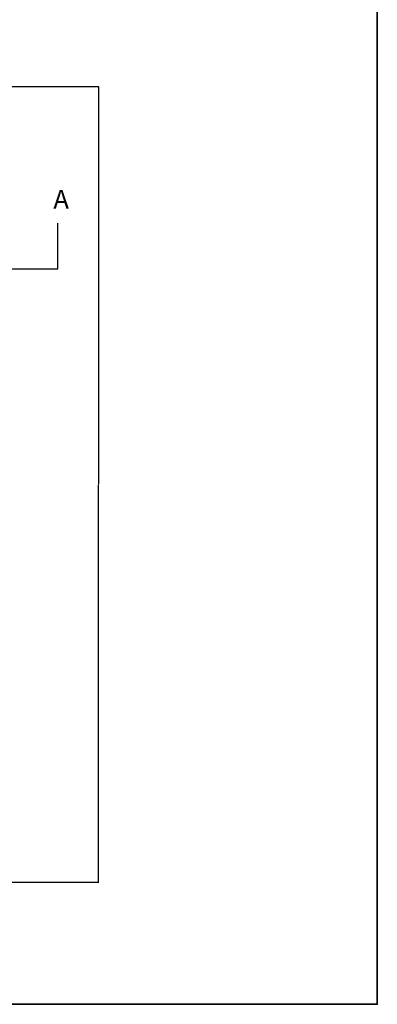
# Model space of a CAD drawing. Units: inches. Extents: x 1832 to 2989, y 1644 to 2902.
# Tile 6 of 8: x 2760 to 2989, y 1644 to 2272. Entities that reach past the tile are written whole.
import ezdxf

# ---------------------------------------------------------------- set-up
doc = ezdxf.new("R2010")
doc.units = ezdxf.units.IN
for name, color, linetype, lineweight in [('A-ANNO-DIMS', 2, 'Continuous', 18), ('A-ANNO-SYMB', 3, 'Continuous', 25), ('A-ANNO-TTLB', 7, 'Continuous', 35)]:
    doc.layers.add(name, color=color, linetype=linetype, lineweight=lineweight)
doc.styles.get("Standard").update_dxf_attribs({"font": 'arial.ttf'})
doc.dimstyles.get("Standard").update_dxf_attribs({"dimtxt": 0.18, "dimasz": 0.18, "dimexe": 0.18, "dimexo": 0.0625, "dimgap": 0.09, "dimtad": 0, "dimtih": 1, "dimtoh": 1, "dimdec": 4, "dimzin": 0, "dimdsep": 46, "dimtxsty": 'Standard', "dimcen": 0.09, "dimadec": 0, "dimazin": 0, "dimtfac": 1, "dimtdec": 4, "dimtofl": 0, "dimtmove": 0, "dimatfit": 3, "dimfxl": 1, "dimtolj": 1, "dimtzin": 0, "dimarcsym": 0})

# ---------------------------------------------------------------- blocks, each defined once
blk = doc.blocks.new('*D82')
at = {"layer": 'A-ANNO-DIMS', "color": 0, "lineweight": -2, "transparency": 16777216}
for p, q in [((2754.1, 2229.17), (2811, 2229.17)), ((2810.82, 2228.99), (2810.82, 1975.53)), ((2810.82, 1721.7), (2810.82, 1975.17)), ((2745.1, 1721.52), (2811, 1721.52))]:
    blk.add_line(p, q, dxfattribs=at)
at = {"layer": 'A-ANNO-DIMS', "color": 0, "transparency": 16777216}
for points in [[(2810.79, 2228.99), (2810.85, 2228.99), (2810.82, 2229.17)], [(2810.79, 1721.7), (2810.85, 1721.7), (2810.82, 1721.52)]]:
    blk.add_solid(points, dxfattribs=at)
at = {"layer": 'Defpoints', "color": 0, "transparency": 16777216}
for p in [(2754.04, 2229.17), (2810.82, 2229.17), (2745.04, 1721.52)]:
    blk.add_point(p, dxfattribs=at)
at = {"layer": 'A-ANNO-DIMS', "color": 0, "transparency": 16777216, "insert": (2810.82, 1975.35), "char_height": 0.18, "attachment_point": 5}
blk.add_mtext('\\A1;507.6', dxfattribs=at)

msp = doc.modelspace()

# ---------------------------------------------------------------- linework, layer by layer
at = {"layer": 'A-ANNO-SYMB'}
for p, q in [((2784.8213, 2112.9108), (2784.8213, 2142.0788)), ((2379.819, 2112.9108), (2784.8213, 2112.9108))]:
    msp.add_line(p, q, dxfattribs=at)
at = {"layer": 'A-ANNO-TTLB'}
msp.add_lwpolyline([(1831.6677, 2901.9044), (2988.9144, 2901.9044), (2988.9144, 1643.5851), (1831.6677, 1643.5851)], close=True, dxfattribs=at)

# ---------------------------------------------------------------- texts
at = {"layer": 'A-ANNO-SYMB', "insert": (2781.9935, 2163.3108), "char_height": 12, "attachment_point": 1}
msp.add_mtext_dynamic_manual_height_columns('A', width=16.638104, gutter_width=12.5, heights=[0], dxfattribs=at)

# ---------------------------------------------------------------- dimensions: what is measured, and where the dimension line sits
at = {"layer": 'A-ANNO-DIMS'}
dim = msp.add_linear_dim(base=(2810.8213, 2229.1726), p1=(2745.0354, 1721.5243), p2=(2754.0354, 2229.1726), angle=90, dimstyle='Standard', override={"dimdec": 1, "dimlfac": 1, "dimrnd": 0, "dimzin": 0, "dimdsep": 46, "dimlunit": 2}, dxfattribs=at)
dim.commit()
dim.dimension.update_dxf_attribs({"geometry": '*D82', "text_midpoint": (2810.8213, 1975.3484)})

doc.saveas('drawing.dxf')
